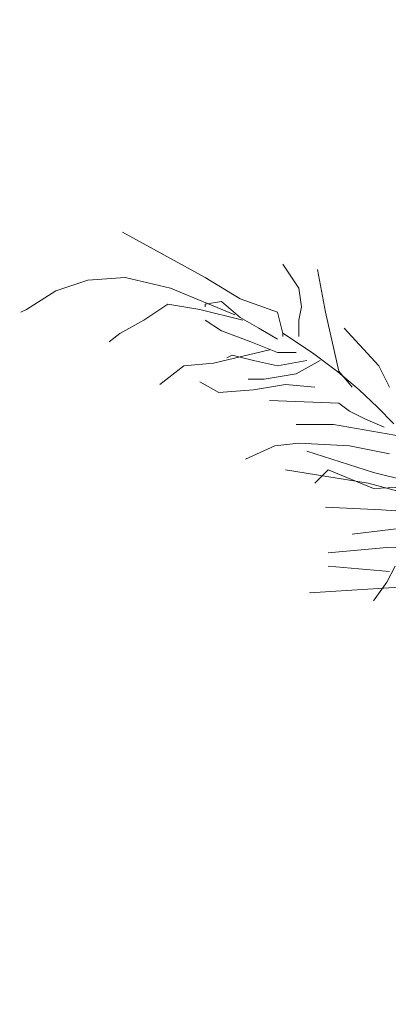
# Model space of a CAD drawing. Units: millimetres. Extents: x 595116 to 630915, y 909473 to 920225.
# Tile 86 of 134: x 629711.176 to 629714.705, y 919275.684 to 919285.103. Entities that reach past the tile are written whole.
import ezdxf

# ---------------------------------------------------------------- set-up
doc = ezdxf.new("R2010")
doc.units = ezdxf.units.MM
doc.layers.add('Dimension', color=3, linetype='Continuous', lineweight=18)
doc.layers.add('L-PLNT', color=85, linetype='Continuous', lineweight=13)
doc.styles.get("Standard").update_dxf_attribs({"font": 'arial.ttf'})
doc.dimstyles.new('ISO-25', dxfattribs={"dimtxt": 9, "dimasz": 6, "dimexe": 1.25, "dimexo": 0.625, "dimtad": 1, "dimlunit": 4, "dimtxsty": 'Standard', "dimcen": 2.5, "dimadec": 0, "dimazin": 0, "dimtfac": 1, "dimtmove": 0, "dimatfit": 3, "dimfxl": 1, "dimarcsym": 0})

# ---------------------------------------------------------------- blocks, each defined once
blk = doc.blocks.new('A$C4FB75ABC')
for p, q in [((0.4999, 4.2779), (0.7111, 4.1621)), ((0.9087, 4.1962), (0.9496, 4.1349)), ((0.9973, 4.1826), (1.0177, 4.0736)), ((0.4114, 4.1553), (0.3296, 4.1281)), ((0.5068, 4.1621), (0.4114, 4.1553)), ((0.6226, 4.1349), (0.5068, 4.1621)), ((0.7111, 4.1621), (0.7997, 4.1076)), ((0.3296, 4.1281), (0.2547, 4.0804)), ((0.7861, 4.0668), (0.6226, 4.1349)), ((0.9496, 4.1349), (0.9564, 4.0872)), ((0.6158, 4.094), (0.5544, 4.0532)), ((0.6975, 4.0804), (0.6158, 4.094)), ((0.752, 4.1008), (0.7111, 4.094)), ((0.7111, 4.094), (0.7111, 4.0872)), ((0.7997, 4.06), (0.752, 4.1008)), ((0.7997, 4.1076), (0.8951, 4.0736)), ((0.2547, 4.0804), (0.241, 4.0736)), ((0.8065, 4.0532), (0.6975, 4.0804)), ((0.8951, 4.0736), (0.9087, 4.0191)), ((0.9564, 4.0872), (0.9496, 4.0532)), ((1.0177, 4.0736), (1.0518, 3.9238)), ((0.5544, 4.0532), (0.4931, 4.0191)), ((0.7111, 4.0532), (0.752, 4.0259)), ((0.8474, 4.0327), (0.7997, 4.06)), ((0.9496, 4.0532), (0.9496, 4.0123)), ((0.4931, 4.0191), (0.4659, 3.9987)), ((0.752, 4.0259), (0.827, 3.9987)), ((0.8951, 4.0055), (0.8474, 4.0327)), ((0.9842, 3.9699), (0.9085, 4.0207)), ((0.9087, 4.0191), (0.9087, 4.0123)), ((1.0654, 4.0327), (1.154, 3.9374)), ((0.827, 3.9987), (0.8951, 3.9715)), ((0.8746, 3.9783), (0.7316, 3.9442)), ((0.8951, 3.9715), (0.9428, 3.9715)), ((1.0487, 3.9217), (0.9842, 3.9699)), ((0.7316, 3.9442), (0.6566, 3.9374)), ((0.7793, 3.9647), (0.7656, 3.9578)), ((0.8338, 3.951), (0.7793, 3.9647)), ((0.8951, 3.9374), (0.8338, 3.951)), ((0.97, 3.951), (0.8951, 3.9374)), ((1.0041, 3.951), (0.9428, 3.917)), ((0.6566, 3.9374), (0.5953, 3.8897)), ((0.9428, 3.917), (0.861, 3.9034)), ((1.1035, 3.8758), (1.0487, 3.9217)), ((1.0518, 3.9238), (1.0858, 3.8829)), ((1.154, 3.9374), (1.1812, 3.8829)), ((0.7452, 3.8693), (0.6975, 3.8966)), ((0.861, 3.9034), (0.8201, 3.9034)), ((0.8338, 3.8761), (0.7452, 3.8693)), ((0.9155, 3.8897), (0.8338, 3.8761)), ((0.9905, 3.8829), (0.9155, 3.8897)), ((1.1506, 3.8319), (1.1035, 3.8758)), ((0.8746, 3.8489), (1.0518, 3.8421)), ((1.0518, 3.8421), (1.079, 3.8217)), ((1.079, 3.8217), (1.1199, 3.8012)), ((1.1917, 3.7897), (1.1506, 3.8319)), ((1.1199, 3.8012), (1.1676, 3.7808)), ((0.9428, 3.7876), (1.0382, 3.7876)), ((1.0382, 3.7876), (1.2698, 3.7467)), ((0.8883, 3.7331), (0.9496, 3.7399)), ((0.9496, 3.7399), (1.079, 3.7331)), ((0.8133, 3.6991), (0.8883, 3.7331)), ((0.97, 3.7195), (1.1403, 3.665)), ((1.079, 3.7331), (1.1812, 3.7127)), ((0.9155, 3.6718), (1.1267, 3.6378)), ((1.0245, 3.6718), (0.9905, 3.6378)), ((1.1403, 3.6242), (1.0245, 3.6718)), ((1.1403, 3.665), (1.2221, 3.6446)), ((1.1267, 3.6378), (1.2017, 3.6174)), ((1.2766, 3.631), (1.1403, 3.6242)), ((1.0177, 3.5765), (1.1608, 3.5697)), ((1.1608, 3.5697), (1.3788, 3.5561)), ((1.0858, 3.5084), (1.2562, 3.5288)), ((1.0245, 3.4608), (1.1744, 3.4744)), ((1.1744, 3.4744), (1.5219, 3.4676)), ((1.0245, 3.4267), (1.1812, 3.4131)), ((1.1949, 3.4267), (1.1744, 3.3858)), ((0.9768, 3.3586), (1.3107, 3.379)), ((1.1744, 3.3858), (1.1403, 3.3382))]:
    blk.add_line(p, q)
blk = doc.blocks.new('*D216')
at = {"layer": 'Defpoints', "color": 0, "transparency": 16777216}
for p in [(629743.5408, 919411.9276), (629505.0408, 919411.8279), (629743.5408, 918832.3776)]:
    blk.add_point(p, dxfattribs=at)
at = {"layer": 'Dimension', "color": 0, "lineweight": -2, "transparency": 16777216}
for p, q in [((629743.5408, 919411.3026), (629743.5408, 918831.1276)), ((629505.0408, 919411.2029), (629505.0408, 918831.1276)), ((629511.0408, 918832.3776), (629737.5408, 918832.3776))]:
    blk.add_line(p, q, dxfattribs=at)
at = {"layer": 'Dimension', "color": 0, "transparency": 16777216}
for points in [[(629511.0408, 918833.3776), (629511.0408, 918831.3776), (629505.0408, 918832.3776)], [(629737.5408, 918833.3776), (629737.5408, 918831.3776), (629743.5408, 918832.3776)]]:
    blk.add_solid(points, dxfattribs=at)
at = {"layer": 'Dimension', "color": 0, "transparency": 16777216, "insert": (629624.2908, 918837.656), "char_height": 9, "attachment_point": 5}
blk.add_mtext('19\'-10 1/2"', dxfattribs=at)

msp = doc.modelspace()

# ---------------------------------------------------------------- block references
at = {"layer": 'L-PLNT', "xscale": 3.753413438031968, "yscale": 3.753413438031968, "zscale": 3.753413438031968}
msp.add_blockref('A$C4FB75ABC', (629710.2837, 919267.0144), dxfattribs=at)

# ---------------------------------------------------------------- dimensions: what is measured, and where the dimension line sits
at = {"layer": 'Dimension'}
dim = msp.add_linear_dim(base=(629743.5408, 918832.3776), p1=(629505.0408, 919411.8279), p2=(629743.5408, 919411.9276), dimstyle='ISO-25', override={"dimdec": 1, "dimlfac": 1, "dimrnd": 0, "dimzin": 1, "dimdsep": 46, "dimlunit": 4, "dimfrac": 2}, dxfattribs=at)
dim.commit()
dim.dimension.update_dxf_attribs({"geometry": '*D216', "text_midpoint": (629624.2908, 918837.656)})

doc.saveas('drawing.dxf')
